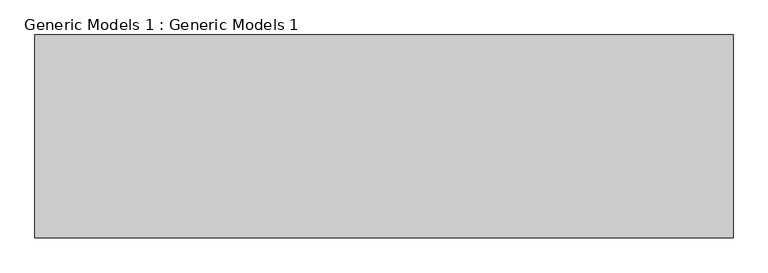
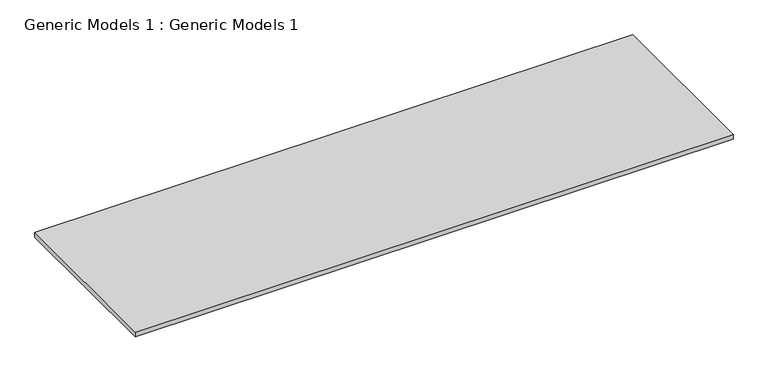
"""IFC4 building model written with IfcOpenShell, lengths in millimetres: proxy geometry, Generic Models 1 : Generic Models 1."""

from ifc_helpers import new_model, si_unit, frame, origin, place, context, project, spatial, polyline, outline, extrude, source, transform, mapped, element, save


def generic_models_1_generic_models_1_070c5cf9(model_context):
    return source(origin(), model_context, "Body", "SweptSolid", [
        extrude(outline(polyline([(-10250.9791129, -13932.5165555), (8037.0208871, -13932.5165555), (8037.0208871, -19248.1924998), (-10250.9791129, -19248.1924998), (-10250.9791129, -13932.5165555)])), frame((0.0, 0.0, -152.4), z_axis=(0.0, 0.0, 1.0), x_axis=(1.0, 0.0, 0.0)), (0.0, 0.0, 1.0), 152.4),
    ])


if __name__ == "__main__":
    model = new_model("IFC4")
    model_context = context("Model", 3, world=origin())
    ifc_project = project(units=[si_unit("LENGTHUNIT", "METRE", prefix="MILLI")], contexts=[model_context])
    site = spatial("IfcSite", under=ifc_project)
    building = spatial("IfcBuilding", under=site)
    placement = place(None, origin())
    generic_models_1_generic_models_1_shape = generic_models_1_generic_models_1_070c5cf9(model_context)
    element("IfcBuildingElementProxy", 1, Name="Generic Models 1 : Generic Models 1", ObjectType="Generic Models 1 : Generic Models 1", at=placement, inside=building, context=model_context, shape_type="MappedRepresentation", body=[
        mapped(generic_models_1_generic_models_1_shape, transform((0.0, 0.0, 0.0), x_axis=(1.0, 0.0, 0.0), y_axis=(0.0, 1.0, 0.0), z_axis=(0.0, 0.0, 1.0))),
    ])
    save(model, "model.ifc")
